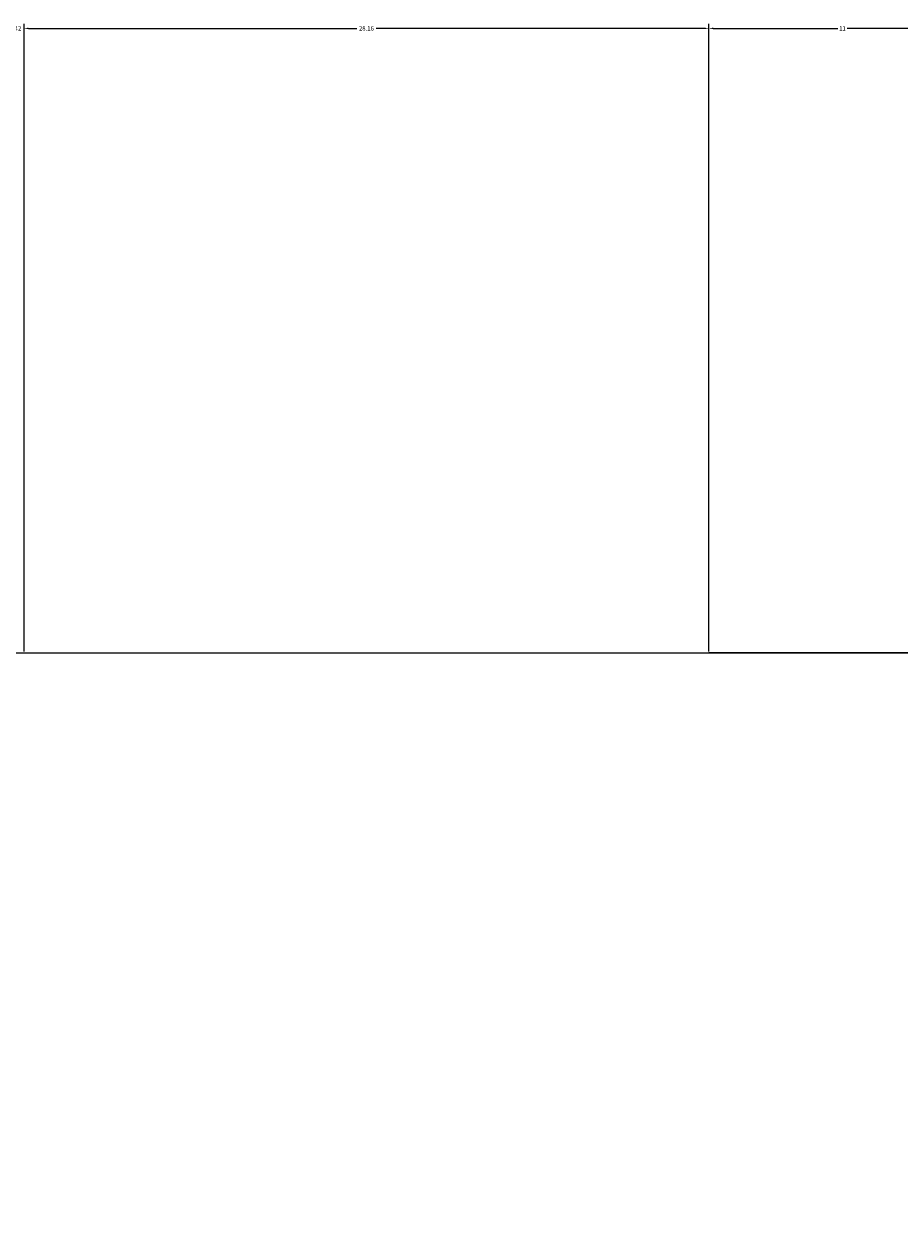
# Model space of a CAD drawing. Units: millimetres. Extents: x -136 to 10, y 158 to 257.
# Tile 5 of 6: x -62 to -26, y 208 to 257. Entities that reach past the tile are written whole.
import ezdxf

# ---------------------------------------------------------------- set-up
doc = ezdxf.new("R2010")
doc.units = ezdxf.units.MM
doc.layers.add('M-CONS', color=8, linetype='Continuous', lineweight=18)
doc.layers.add('M-DIMS', color=2, linetype='Continuous', lineweight=18)
doc.styles.get("Standard").update_dxf_attribs({"font": 'arial.ttf'})
doc.dimstyles.get("Standard").update_dxf_attribs({"dimtxt": 0.18, "dimasz": 0.18, "dimexe": 0.18, "dimexo": 0.0625, "dimgap": 0.09, "dimtad": 0, "dimtih": 1, "dimtoh": 1, "dimdec": 4, "dimzin": 0, "dimdsep": 46, "dimtxsty": 'Standard', "dimcen": 0.09, "dimadec": 0, "dimazin": 0, "dimtfac": 1, "dimtdec": 4, "dimtofl": 0, "dimtmove": 0, "dimatfit": 3, "dimfxl": 1, "dimtolj": 1, "dimtzin": 0, "dimarcsym": 0})

# ---------------------------------------------------------------- blocks, each defined once
blk = doc.blocks.new('*D1')
at = {"layer": 'Defpoints', "color": 0, "transparency": 16777216}
for p in [(-126, 231.107), (0, 231.107), (0, 158.407)]:
    blk.add_point(p, dxfattribs=at)
at = {"layer": 'M-DIMS', "color": 0, "lineweight": -2, "transparency": 16777216}
for p, q in [((-126, 231.044), (-126, 158.227)), ((0, 231.044), (0, 158.227)), ((-125.82, 158.407), (-63.28, 158.407)), ((-0.18, 158.407), (-62.72, 158.407))]:
    blk.add_line(p, q, dxfattribs=at)
at = {"layer": 'M-DIMS', "color": 0, "transparency": 16777216}
for points in [[(-125.82, 158.437), (-125.82, 158.377), (-126, 158.407)], [(-0.18, 158.437), (-0.18, 158.377), (0, 158.407)]]:
    blk.add_solid(points, dxfattribs=at)
at = {"layer": 'M-DIMS', "color": 0, "transparency": 16777216, "insert": (-63, 158.407), "char_height": 0.18, "attachment_point": 5}
blk.add_mtext('\\A1;126', dxfattribs=at)
blk = doc.blocks.new('*D2')
at = {"layer": 'Defpoints', "color": 0, "transparency": 16777216}
for p in [(0, 247.107), (9.7, 247.107), (-62.158, 168.107)]:
    blk.add_point(p, dxfattribs=at)
at = {"layer": 'M-DIMS', "color": 0, "lineweight": -2, "transparency": 16777216}
for p, q in [((0.062, 247.107), (9.88, 247.107)), ((9.7, 246.927), (9.7, 207.789)), ((9.7, 168.287), (9.7, 207.425)), ((-62.095, 168.107), (9.88, 168.107))]:
    blk.add_line(p, q, dxfattribs=at)
at = {"layer": 'M-DIMS', "color": 0, "transparency": 16777216}
for points in [[(9.67, 246.927), (9.73, 246.927), (9.7, 247.107)], [(9.67, 168.287), (9.73, 168.287), (9.7, 168.107)]]:
    blk.add_solid(points, dxfattribs=at)
at = {"layer": 'M-DIMS', "color": 0, "transparency": 16777216, "insert": (9.7, 207.607), "char_height": 0.18, "attachment_point": 5}
blk.add_mtext('\\A1;79', dxfattribs=at)
blk = doc.blocks.new('*D3')
at = {"layer": 'Defpoints', "color": 0, "transparency": 16777216}
for p in [(-126, 231.107), (-135.7, 168.107), (-62.158, 168.107)]:
    blk.add_point(p, dxfattribs=at)
at = {"layer": 'M-DIMS', "color": 0, "lineweight": -2, "transparency": 16777216}
for p, q in [((-126.062, 231.107), (-135.88, 231.107)), ((-135.7, 230.927), (-135.7, 199.789)), ((-135.7, 168.287), (-135.7, 199.425)), ((-62.22, 168.107), (-135.88, 168.107))]:
    blk.add_line(p, q, dxfattribs=at)
at = {"layer": 'M-DIMS', "color": 0, "transparency": 16777216}
for points in [[(-135.73, 230.927), (-135.67, 230.927), (-135.7, 231.107)], [(-135.73, 168.287), (-135.67, 168.287), (-135.7, 168.107)]]:
    blk.add_solid(points, dxfattribs=at)
at = {"layer": 'M-DIMS', "color": 0, "transparency": 16777216, "insert": (-135.7, 199.607), "char_height": 0.18, "attachment_point": 5}
blk.add_mtext('\\A1;63', dxfattribs=at)
blk = doc.blocks.new('*D9')
at = {"layer": 'Defpoints', "color": 0, "transparency": 16777216}
for p in [(-62.157998, 256.806753), (-63, 231.106753), (-62.157998, 231.106753)]:
    blk.add_point(p, dxfattribs=at)
at = {"layer": 'M-DIMS', "color": 0, "lineweight": -2, "transparency": 16777216}
for p, q in [((-63.18, 256.806753), (-63.36, 256.806753)), ((-63, 231.169253), (-63, 256.986753)), ((-62.157998, 231.169253), (-62.157998, 256.986753)), ((-61.977998, 256.806753), (-61.797998, 256.806753))]:
    blk.add_line(p, q, dxfattribs=at)
at = {"layer": 'M-DIMS', "color": 0, "transparency": 16777216}
for points in [[(-63.18, 256.836753), (-63.18, 256.776753), (-63, 256.806753)], [(-61.977998, 256.836753), (-61.977998, 256.776753), (-62.157998, 256.806753)]]:
    blk.add_solid(points, dxfattribs=at)
at = {"layer": 'M-DIMS', "color": 0, "transparency": 16777216, "insert": (-62.578999, 256.806753), "char_height": 0.18, "attachment_point": 5}
blk.add_mtext('\\A1;0.842', dxfattribs=at)
blk = doc.blocks.new('*D10')
at = {"layer": 'Defpoints', "color": 0, "transparency": 16777216}
for p in [(-34, 256.807), (-62.158, 231.107), (-34, 231.107)]:
    blk.add_point(p, dxfattribs=at)
at = {"layer": 'M-DIMS', "color": 0, "lineweight": -2, "transparency": 16777216}
for p, q in [((-62.158, 231.169), (-62.158, 256.987)), ((-61.978, 256.807), (-48.474, 256.807)), ((-34.18, 256.807), (-47.684, 256.807)), ((-34, 231.169), (-34, 256.987))]:
    blk.add_line(p, q, dxfattribs=at)
at = {"layer": 'M-DIMS', "color": 0, "transparency": 16777216}
for points in [[(-61.978, 256.837), (-61.978, 256.777), (-62.158, 256.807)], [(-34.18, 256.837), (-34.18, 256.777), (-34, 256.807)]]:
    blk.add_solid(points, dxfattribs=at)
at = {"layer": 'M-DIMS', "color": 0, "transparency": 16777216, "insert": (-48.079, 256.807), "char_height": 0.18, "attachment_point": 5}
blk.add_mtext('\\A1;28.16', dxfattribs=at)
blk = doc.blocks.new('*D11')
at = {"layer": 'Defpoints', "color": 0, "transparency": 16777216}
for p in [(-23, 256.807), (-34, 231.107), (-23, 231.107)]:
    blk.add_point(p, dxfattribs=at)
at = {"layer": 'M-DIMS', "color": 0, "lineweight": -2, "transparency": 16777216}
for p, q in [((-34, 231.169), (-34, 256.987)), ((-33.82, 256.807), (-28.693, 256.807)), ((-23.18, 256.807), (-28.307, 256.807)), ((-23, 231.169), (-23, 256.987))]:
    blk.add_line(p, q, dxfattribs=at)
at = {"layer": 'M-DIMS', "color": 0, "transparency": 16777216}
for points in [[(-33.82, 256.837), (-33.82, 256.777), (-34, 256.807)], [(-23.18, 256.837), (-23.18, 256.777), (-23, 256.807)]]:
    blk.add_solid(points, dxfattribs=at)
at = {"layer": 'M-DIMS', "color": 0, "transparency": 16777216, "insert": (-28.5, 256.807), "char_height": 0.18, "attachment_point": 5}
blk.add_mtext('\\A1;11', dxfattribs=at)

msp = doc.modelspace()

# ---------------------------------------------------------------- linework, layer by layer
at = {"layer": 'M-CONS'}
msp.add_line((-63, 231.1068, 128.8035), (-32, 231.1068, 128.8035), dxfattribs=at)
at = {"layer": 'M-CONS', "extrusion": (0, -1, 0)}
msp.add_circle((-18, 98.8035, -231.1068), 16, dxfattribs=at)

# ---------------------------------------------------------------- dimensions: what is measured, and where the dimension line sits
at = {"layer": 'M-DIMS'}
for base, p1, p2, override, picture, middle in [((-62.158, 256.8068), (-63, 231.1068), (-62.158, 231.1068), {"dimdec": 3, "dimlfac": 1, "dimrnd": 0, "dimzin": 0, "dimdsep": 46, "dimlunit": 2}, '*D9', (-62.579, 256.8068)), ((-34, 256.8068), (-62.158, 231.1068), (-34, 231.1068), {"dimdec": 2, "dimlfac": 1, "dimrnd": 0, "dimzin": 0, "dimdsep": 46, "dimlunit": 2}, '*D10', (-48.079, 256.8068)), ((-23, 256.8068), (-34, 231.1068), (-23, 231.1068), {"dimdec": 0, "dimlfac": 1, "dimrnd": 0, "dimzin": 0, "dimdsep": 46, "dimlunit": 2}, '*D11', (-28.5, 256.8068)), ((0, 158.4068), (-126, 231.1068), (0, 231.1068), {"dimdec": 0, "dimlfac": 1, "dimrnd": 0, "dimzin": 0, "dimdsep": 46, "dimlunit": 2}, '*D1', (-63, 158.4068))]:
    dim = msp.add_linear_dim(base=base, p1=p1, p2=p2, dimstyle='Standard', override=override, dxfattribs=at)
    dim.commit()
    dim.dimension.update_dxf_attribs({"geometry": picture, "text_midpoint": middle})
for base, p1, p2, picture, middle in [((9.7, 247.1068), (-62.158, 168.1068), (0, 247.1068), '*D2', (9.7, 207.6068)), ((-135.7, 168.1068), (-126, 231.1068), (-62.158, 168.1068), '*D3', (-135.7, 199.6068))]:
    dim = msp.add_linear_dim(base=base, p1=p1, p2=p2, angle=90, dimstyle='Standard', override={"dimdec": 0, "dimlfac": 1, "dimrnd": 0, "dimzin": 0, "dimdsep": 46, "dimlunit": 2}, dxfattribs=at)
    dim.commit()
    dim.dimension.update_dxf_attribs({"geometry": picture, "text_midpoint": middle})

doc.saveas('drawing.dxf')
